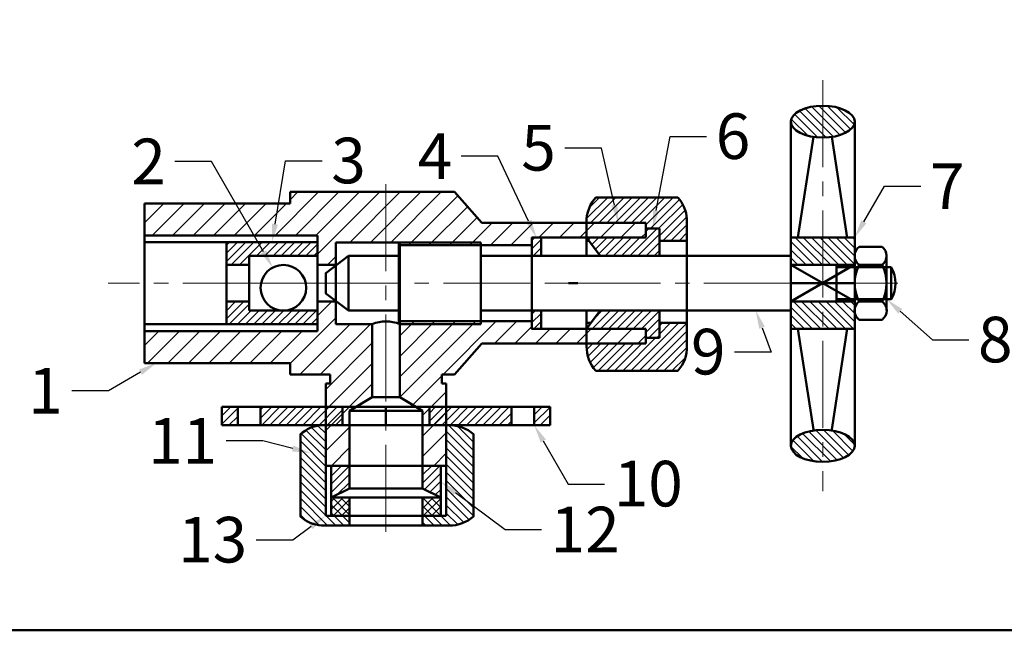
# Model space of a CAD drawing. Units: millimetres. Extents: x 123 to 731, y 468 to 864.
# Tile 2 of 5: x 328 to 544, y 468 to 602. Entities that reach past the tile are written whole.
import ezdxf
from ezdxf import colors
from ezdxf.entities.mleader import LeaderData, LeaderLine
from ezdxf.math import Vec2, Vec3

# ---------------------------------------------------------------- set-up
doc = ezdxf.new("R2010")
doc.units = ezdxf.units.MM
doc.linetypes.add('CENTER2', pattern=[28.575, 19.05, -3.175, 3.175, -3.175])
for name, color, linetype, lineweight in [('M-CNTR', 1, 'CENTER2', 18), ('M-HATC', 8, 'Continuous', 18), ('M-OUTL', 7, 'Continuous', 50), ('M-TEXT', 3, 'Continuous', 25)]:
    doc.layers.add(name, color=color, linetype=linetype, lineweight=lineweight)
doc.styles.get("Standard").update_dxf_attribs({"font": 'arial.ttf'})
pattern_1 = [(45, (-48.4416, -233.5905), (-0.8980256, 0.8980256), [])]
pattern_2 = [(135, (832.0712, 132.0536), (-0.8980256, -0.8980256), [])]
pattern_3 = [(45, (832.0712, 132.0536), (-0.8980256, 0.8980256), [])]

# ---------------------------------------------------------------- blocks, each defined once
blk = doc.blocks.new('*U26')
at = {"layer": 'M-CNTR', "color": 0, "transparency": 16777216}
blk.add_line((44.29, 0), (-105.45, 0), dxfattribs=at)
blk = doc.blocks.new('*U40')
at = {"layer": 'M-CNTR', "color": 0, "transparency": 16777216}
blk.add_line((6, 0), (-6, 0), dxfattribs=at)
blk = doc.blocks.new('*U42')
at = {"layer": 'M-CNTR', "color": 0, "transparency": 16777216}
blk.add_line((4.5, 0), (-4.5, 0), dxfattribs=at)
blk = doc.blocks.new('*U46')
at = {"layer": 'M-CNTR', "color": 0, "transparency": 16777216}
blk.add_line((0, -5.5), (0, 73.5), dxfattribs=at)
blk = doc.blocks.new('*U71')
at = {"layer": 'M-CNTR', "color": 0, "transparency": 16777216}
blk.add_line((13.5, 0), (-13.5, 0), dxfattribs=at)
blk = doc.blocks.new('*U83')
at = {"layer": 'M-CNTR', "color": 0, "transparency": 16777216}
blk.add_line((0, 53.48), (0, -36.6), dxfattribs=at)
blk = doc.blocks.new('HEX-NUT')
for p, q in [((6.02, 16), (1.02, 16)), ((1.02, 12), (6.02, 12)), ((1.02, 4), (6.02, 4)), ((1.02, 0), (6.02, 0))]:
    blk.add_line(p, q)
for centre, radius, start, end in [((2.47, 14), 2.47, 125.9888, 234.0112), ((4.57, 14), 2.47, 305.9888, 54.0112), ((8.52, 8), 8.5, 151.9275, 208.0725), ((-1.48, 8), 8.5, 331.9275, 28.0725), ((2.52, 2), 2.5, 126.8697, 233.1303), ((4.52, 2), 2.5, 306.8697, 53.1303)]:
    blk.add_arc(centre, radius, start, end)

msp = doc.modelspace()

# ---------------------------------------------------------------- hatches: boundary and pattern name
at = {"layer": 'M-HATC'}
h = msp.add_hatch(dxfattribs=at)
h.set_pattern_fill('ANSI31', color=256, scale=0.4, angle=-90)
h.set_pattern_definition([(315, (-204.5358, 1199.6268), (0.8980256, 0.8980256), [])])
edge = h.paths.add_edge_path()
edge.add_ellipse((504.0866, 579.9567), major_axis=(-7, 0), ratio=0.5, start_angle=90, end_angle=270)
edge.add_line((504.0866, 583.4567), (504.0866, 576.4567))
edge = h.paths.add_edge_path()
edge.add_ellipse((504.0866, 579.9567), major_axis=(-7, 0), ratio=0.5, start_angle=270, end_angle=450)
edge.add_line((504.0866, 576.4567), (504.0866, 583.4567))
h.paths.add_polyline_path([(511.0866, 548.5375), (511.0866, 554.5375), (504.0866, 554.5375), (504.0866, 548.5375)])
h.paths.add_polyline_path([(504.0866, 548.5375), (504.0866, 554.5375), (497.0866, 554.5375), (497.0866, 548.5375)])
h.paths.add_polyline_path([(511.0866, 534.5375), (511.0866, 540.5375), (504.0866, 540.5375), (504.0866, 534.5375)])
h.paths.add_polyline_path([(504.0866, 540.5375), (497.0866, 540.5375), (497.0866, 534.5375), (504.0866, 534.5375)])
edge = h.paths.add_edge_path()
edge.add_ellipse((504.0866, 508.902), major_axis=(-7, 0), ratio=0.5, start_angle=90, end_angle=270)
edge.add_line((504.0866, 512.402), (504.0866, 505.402))
edge = h.paths.add_edge_path()
edge.add_ellipse((504.0866, 508.902), major_axis=(-7, 0), ratio=0.5, start_angle=270, end_angle=450)
edge.add_line((504.0866, 505.402), (504.0866, 512.402))
h = msp.add_hatch(dxfattribs=at)
h.set_pattern_fill('ANSI31', color=256)
h.set_pattern_definition([(45, (832.0712, 132.0536), (-2.245064, 2.245064), [])])
h.paths.add_polyline_path([(411.2945, 519.5375), (416.2945, 516.5375), (416.2945, 504.5375), (421.5145, 504.5375), (421.5145, 522.5375), (420.5145, 522.5375), (420.5145, 524.5375), (423.2945, 524.5375), (429.2945, 531.3175), (440.2945, 531.3175), (465.2945, 531.3175), (465.2945, 534.5375), (440.2945, 534.5375), (440.2945, 536.2075), (411.2945, 536.2075), (411.2945, 535.5746)])
h.paths.add_polyline_path([(405.2945, 535.5746), (397.2945, 535.5746), (397.2945, 540.5375), (393.2945, 540.5375), (393.2945, 534.0575), (355.2945, 534.0575), (355.2945, 527.0375), (387.2945, 527.0375), (387.2945, 524.5375), (396.0745, 524.5375), (396.0745, 522.5375), (395.0745, 522.5375), (395.0745, 504.5375), (400.2945, 504.5375), (400.2945, 516.5375), (405.2945, 519.5375)])
h.paths.add_polyline_path([(387.2945, 564.5375), (387.2945, 562.0375), (355.2945, 562.0375), (355.2945, 555.0175), (393.2945, 555.0175), (393.2945, 548.5375), (397.2945, 548.5375), (397.2945, 553.5004), (411.2945, 553.5004), (411.2945, 552.8675), (440.2945, 552.8675), (440.2945, 554.5375), (465.2945, 554.5375), (465.2945, 557.7575), (440.2945, 557.7575), (429.2945, 557.7575), (423.2945, 564.5375)])
h = msp.add_hatch(dxfattribs=at)
h.set_pattern_fill('ANSI31', color=256, scale=0.4)
h.set_pattern_definition(pattern_3)
h.paths.add_polyline_path([(474.2945, 530.428), (474.2945, 535.8212), (468.2945, 535.8212), (468.2945, 532.5375), (465.2945, 532.5375), (465.2945, 531.3175), (452.2945, 531.3175), (452.2945, 530.428, 0.17944614), (454.2945, 525.3212), (472.2945, 525.3212, 0.17944614)])
h.paths.add_polyline_path([(472.2945, 563.3212), (454.2945, 563.3212, 0.16687276), (452.2945, 558.647), (452.2945, 557.7575), (465.2945, 557.7575), (465.2945, 556.5375), (468.2945, 556.5375), (468.2945, 553.8462), (474.2945, 553.8462), (474.2945, 558.647, 0.16687276)])
h = msp.add_hatch(dxfattribs=at)
h.set_pattern_fill('ANSI31', color=256, scale=0.4)
h.set_pattern_definition([(45, (-79.6213, -197.3759), (-0.8980256, 0.8980256), [])])
h.paths.add_polyline_path([(452.2945, 554.5375), (455.2945, 550.5375), (468.2945, 550.5375), (468.2945, 556.5375), (465.2945, 556.5375), (465.2945, 554.5375)])
h = msp.add_hatch(dxfattribs=at)
h.set_pattern_fill('ANSI31', color=256, scale=0.4)
h.set_pattern_definition([(45, (7.4622, -127.2527), (-0.8980256, 0.8980256), [])])
h.paths.add_polyline_path([(373.2945, 548.5375), (378.2945, 548.5375), (378.2945, 550.5375), (393.2945, 550.5375), (393.2945, 553.5375), (373.2945, 553.5375)])
h.paths.add_polyline_path([(393.2945, 535.5375), (393.2945, 538.5375), (378.2945, 538.5375), (378.2945, 540.5375), (373.2945, 540.5375), (373.2945, 535.5375)])
h = msp.add_hatch(dxfattribs=at)
h.set_pattern_fill('ANSI31', color=256, scale=0.4)
h.set_pattern_definition(pattern_3)
h.paths.add_polyline_path([(440.2945, 550.5375), (442.2945, 550.5375), (442.2945, 554.5375), (440.2945, 554.5375)])
h.paths.add_polyline_path([(442.2945, 538.5375), (440.2945, 538.5375), (440.2945, 534.5375), (442.2945, 534.5375)])
h = msp.add_hatch(dxfattribs=at)
h.set_pattern_fill('ANSI31', color=256, scale=0.4)
h.set_pattern_definition([(45, (-161.0183, -242.7467), (-0.8980256, 0.8980256), [])])
h.paths.add_polyline_path([(452.813, 553.8462), (452.2945, 554.5375), (452.2945, 553.8462)])
h = msp.add_hatch(dxfattribs=at)
h.set_pattern_fill('ANSI31', color=256, scale=0.4)
h.set_pattern_definition([(45, (835.1768, 97.1788), (-0.8980256, 0.8980256), [])])
h.paths.add_polyline_path([(455.2945, 538.5375), (452.2945, 534.5375), (465.2945, 534.5375), (465.2945, 532.5375), (468.2945, 532.5375), (468.2945, 538.5375)])
h = msp.add_hatch(dxfattribs=at)
h.set_pattern_fill('ANSI31', color=256, scale=0.4)
h.set_pattern_definition([(45, (834.237, 76.9075), (-0.8980256, 0.8980256), [])])
h.paths.add_polyline_path([(452.2945, 534.5375), (453.2574, 535.8212), (452.2945, 535.8212)])
h = msp.add_hatch(dxfattribs=at)
h.set_pattern_fill('ANSI31', color=256, scale=0.4)
h.set_pattern_definition([(45, (-72.056, -58.2177), (-0.8980256, 0.8980256), [])])
h.paths.add_polyline_path([(375.7945, 517.4172), (372.2945, 517.4172), (372.2945, 513.4172), (375.7945, 513.4172)])
h.paths.add_polyline_path([(398.7695, 513.4172), (398.7695, 517.4172), (380.7945, 517.4172), (380.7945, 513.4172)])
h.paths.add_polyline_path([(435.7945, 513.4172), (435.7945, 517.4172), (417.8195, 517.4172), (417.8195, 513.4172)])
h.paths.add_polyline_path([(440.7945, 513.4172), (444.2945, 513.4172), (444.2945, 517.4172), (440.7945, 517.4172)])
h = msp.add_hatch(dxfattribs=at)
h.set_pattern_fill('ANSI31', color=256, scale=0.4, angle=90)
h.set_pattern_definition(pattern_2)
h.paths.add_polyline_path([(395.0745, 504.5375), (395.0745, 513.4172), (394.1851, 513.4172, 0.16687276), (389.5108, 511.4172), (389.5108, 493.4172, 0.16687276), (394.1851, 491.4172), (400.2945, 491.4172), (400.2945, 493.5375), (396.2945, 493.5375), (395.0745, 493.5375)])
h.paths.add_polyline_path([(421.5145, 493.5375), (420.2945, 493.5375), (416.2945, 493.5375), (416.2945, 491.4172), (422.404, 491.4172, 0.17944614), (427.5108, 493.4172), (427.5108, 511.4172, 0.20874254), (421.5145, 513.3831), (421.5145, 504.5375)])
h = msp.add_hatch(dxfattribs=at)
h.set_pattern_fill('ANSI31', color=256, scale=0.4)
h.set_pattern_definition([(45, (926.4336, -118.8602), (-0.8980256, 0.8980256), [])])
h.paths.add_polyline_path([(400.2945, 504.5375), (396.2945, 504.5375), (396.2945, 497.5375), (400.2945, 499.5375)])
h.paths.add_polyline_path([(420.2945, 504.5375), (416.2945, 504.5375), (416.2945, 499.5375), (420.2945, 497.5375)])
h = msp.add_hatch(dxfattribs=at)
h.set_pattern_fill('ANSI31', color=256, scale=0.4)
h.set_pattern_definition(pattern_1)
h.paths.add_polyline_path([(396.2945, 497.5375), (400.2945, 497.5375), (400.2945, 493.5375), (396.2945, 493.5375)])
h = msp.add_hatch(dxfattribs=at)
h.set_pattern_fill('ANSI31', color=256, scale=0.4, angle=90)
h.set_pattern_definition(pattern_2)
h.paths.add_polyline_path([(400.2945, 497.5375), (396.2945, 497.5375), (396.2945, 493.5375), (400.2945, 493.5375)])
h.paths.add_polyline_path([(420.2945, 497.5375), (416.2945, 497.5375), (416.2945, 493.5375), (420.2945, 493.5375)])
h = msp.add_hatch(dxfattribs=at)
h.set_pattern_fill('ANSI31', color=256, scale=0.4)
h.set_pattern_definition(pattern_1)
h.paths.add_polyline_path([(416.2945, 493.5375), (420.2945, 493.5375), (420.2945, 497.5375), (416.2945, 497.5375)])

# ---------------------------------------------------------------- linework, layer by layer
at = {"layer": 'M-OUTL'}
for p, q in [((497.0866, 544.5375), (497.0866, 579.9567)), ((511.0866, 579.9567), (511.0866, 508.902)), ((502.0866, 576.6026), (498.615, 554.5375)), ((506.0873, 576.5936), (509.4596, 554.5131)), ((387.2945, 562.0375), (387.2945, 564.5375)), ((387.2945, 564.5375), (423.2945, 564.5375)), ((429.2945, 557.7575), (423.2945, 564.5375)), ((355.2945, 562.0375), (355.2945, 555.0175)), ((355.2945, 562.0375), (387.2945, 562.0375)), ((472.2945, 563.3212), (454.2945, 563.3212)), ((440.2945, 557.7575), (429.2945, 557.7575)), ((465.2945, 557.7575), (440.2945, 557.7575)), ((452.2945, 558.647), (452.2945, 550.5375)), ((465.2945, 556.5375), (465.2945, 557.7575)), ((474.2945, 530.428), (474.2945, 558.647)), ((393.2945, 555.0175), (355.2945, 555.0175)), ((355.2945, 555.0175), (355.2945, 534.0575)), ((393.2945, 555.0175), (393.2945, 548.5375)), ((468.2945, 556.5375), (465.2945, 556.5375)), ((465.2945, 556.5375), (465.2945, 554.5375)), ((468.2945, 550.5375), (468.2945, 556.5375)), ((373.2945, 553.5375), (355.2945, 553.5375)), ((373.2945, 553.5375), (373.2945, 535.5375)), ((393.2945, 553.5375), (373.2945, 553.5375)), ((393.2945, 535.5375), (393.2945, 553.5375)), ((397.2945, 553.5004), (397.2945, 535.5746)), ((411.2945, 553.5004), (397.2945, 553.5004)), ((411.0866, 553.5004), (411.0866, 535.5746)), ((429.0866, 553.5004), (411.0866, 553.5004)), ((411.2945, 553.5004), (411.2945, 544.5375)), ((440.2945, 552.8675), (411.2945, 552.8675)), ((411.2945, 544.5375), (411.2945, 552.8675)), ((440.2945, 554.5375), (440.2945, 534.5375)), ((465.2945, 554.5375), (440.2945, 554.5375)), ((452.2945, 554.5375), (452.2945, 550.5375)), ((465.2945, 554.5375), (452.2945, 554.5375)), ((455.2945, 550.5375), (452.2945, 554.5375)), ((452.2945, 553.8462), (452.813, 553.8462)), ((452.2945, 550.5375), (452.2945, 553.8462)), ((468.2945, 553.8462), (474.2945, 553.8462)), ((497.0866, 554.5375), (511.0866, 554.5375)), ((511.0866, 550.8457), (511.0866, 538.5333)), ((518.0866, 538.5333), (518.0866, 550.8457)), ((373.2945, 548.5375), (378.2945, 548.5375)), ((393.2945, 550.5375), (378.2945, 550.5375)), ((378.2945, 550.5375), (378.2945, 538.5375)), ((397.2945, 548.5375), (393.2945, 548.5375)), ((393.2945, 548.5375), (393.2945, 540.5375)), ((397.2945, 548.5375), (397.2945, 540.5375)), ((411.0866, 550.5375), (400.0866, 550.5375)), ((448.3346, 550.5375), (450.3346, 550.5375)), ((452.2945, 550.5375), (468.2945, 550.5375)), ((497.0866, 548.5375), (511.0866, 548.5375)), ((497.0866, 540.5375), (510.943, 548.5375)), ((497.0866, 548.5375), (511.0866, 540.5375)), ((411.2945, 544.5375), (411.2945, 536.2075)), ((411.2945, 535.5746), (411.2945, 544.5375)), ((448.3346, 544.5375), (450.3346, 544.5375)), ((497.0866, 508.902), (497.0866, 544.5375)), ((497.0866, 544.5375), (511.0866, 544.5375)), ((373.2945, 540.5375), (378.2945, 540.5375)), ((393.2945, 540.5375), (397.2945, 540.5375)), ((393.2945, 534.0575), (393.2945, 540.5375)), ((497.0866, 540.5375), (511.0866, 540.5375)), ((378.2945, 538.5375), (393.2945, 538.5375)), ((448.3346, 538.5375), (450.3346, 538.5375)), ((452.2945, 538.5375), (468.2945, 538.5375)), ((452.2945, 534.5375), (455.2945, 538.5375)), ((452.2945, 538.5375), (452.2945, 530.428)), ((452.2945, 538.5375), (452.2945, 534.5375)), ((468.2945, 532.5375), (468.2945, 538.5375)), ((405.2945, 535.5746), (397.2945, 535.5746)), ((405.2945, 535.5746), (405.2945, 519.5375)), ((440.2945, 536.2075), (411.2945, 536.2075)), ((411.2945, 535.5746), (411.2945, 519.5375)), ((429.0866, 535.5746), (411.2945, 535.5746)), ((452.2945, 535.8212), (453.2574, 535.8212)), ((468.2945, 535.8212), (474.2945, 535.8212)), ((373.2945, 535.5375), (355.2945, 535.5375)), ((355.2945, 534.0575), (393.2945, 534.0575)), ((355.2945, 527.0375), (355.2945, 534.0575)), ((373.2945, 535.5375), (393.2945, 535.5375)), ((465.2945, 534.5375), (440.2945, 534.5375)), ((452.2945, 534.5375), (465.2945, 534.5375)), ((465.2945, 534.5375), (465.2945, 532.5375)), ((497.0866, 534.5375), (511.0866, 534.5375)), ((502.0866, 512.4723), (498.615, 534.5375)), ((506.0873, 512.4813), (509.4596, 534.5619)), ((429.2945, 531.3175), (423.2945, 524.5375)), ((440.2945, 531.3175), (429.2945, 531.3175)), ((465.2945, 531.3175), (440.2945, 531.3175)), ((465.2945, 531.3175), (440.2945, 531.3175)), ((465.2945, 532.5375), (468.2945, 532.5375)), ((465.2945, 531.3175), (465.2945, 532.5375)), ((355.2945, 527.0375), (387.2945, 527.0375)), ((387.2945, 527.0375), (387.2945, 524.5375)), ((454.2945, 525.3212), (472.2945, 525.3212)), ((387.2945, 524.5375), (396.0745, 524.5375)), ((395.0745, 524.5375), (396.0745, 524.5375)), ((396.0745, 524.5375), (396.0745, 522.5375)), ((420.5145, 524.5375), (420.5145, 522.5375)), ((420.5145, 524.5375), (423.2945, 524.5375)), ((395.0745, 504.5375), (395.0745, 522.5375)), ((396.0745, 522.5375), (395.0745, 522.5375)), ((420.5145, 522.5375), (421.5145, 522.5375)), ((421.5145, 504.5375), (421.5145, 522.5375)), ((405.2945, 519.5375), (400.2945, 516.5375)), ((405.2945, 519.5375), (411.2945, 519.5375)), ((411.2945, 519.5375), (416.2945, 516.5375)), ((444.2945, 517.4172), (372.2945, 517.4172)), ((372.2945, 517.4172), (372.2945, 513.4172)), ((375.7945, 513.4172), (375.7945, 517.4172)), ((380.7945, 513.4172), (380.7945, 517.4172)), ((398.7695, 517.4172), (398.7695, 513.4172)), ((416.2945, 516.5375), (400.2945, 516.5375)), ((400.2945, 516.5375), (400.2945, 504.5375)), ((408.2945, 517.4172), (408.2945, 513.4172)), ((416.2945, 504.5375), (416.2945, 516.5375)), ((417.8195, 517.4172), (417.8195, 513.4172)), ((435.7945, 513.4172), (435.7945, 517.4172)), ((440.7945, 513.4172), (440.7945, 517.4172)), ((444.2945, 513.4172), (444.2945, 517.4172)), ((372.2945, 513.4172), (444.2945, 513.4172)), ((408.2945, 504.5375), (395.0745, 504.5375)), ((395.0745, 504.5375), (395.0745, 493.5375)), ((420.2945, 504.5375), (396.2945, 504.5375)), ((396.2945, 504.5375), (396.2945, 497.5375)), ((400.2945, 504.5375), (416.2945, 504.5375)), ((400.2945, 504.5375), (400.2945, 499.5375)), ((408.2945, 504.5375), (421.5145, 504.5375)), ((416.2945, 504.5375), (416.2945, 499.5375)), ((420.2945, 497.5375), (420.2945, 504.5375)), ((421.5145, 504.5375), (421.5145, 493.5375)), ((400.2945, 499.5375), (396.2945, 497.5375)), ((400.2945, 499.5375), (408.2945, 499.5375)), ((416.2945, 499.5375), (408.2945, 499.5375)), ((416.2945, 499.5375), (420.2945, 497.5375)), ((420.2945, 497.5375), (396.2945, 497.5375)), ((396.2945, 497.5375), (396.2945, 493.5375)), ((396.2945, 497.5375), (420.2945, 497.5375)), ((400.2945, 497.5375), (400.2945, 493.5375)), ((416.2945, 497.5375), (416.2945, 493.5375)), ((420.2945, 493.5375), (420.2945, 497.5375)), ((396.2945, 493.5375), (395.0745, 493.5375)), ((396.2945, 493.5375), (420.2945, 493.5375)), ((400.2945, 493.5375), (400.2945, 491.4172)), ((416.2945, 493.5375), (416.2945, 491.4172)), ((420.2945, 493.5375), (421.5145, 493.5375))]:
    msp.add_line(p, q, dxfattribs=at)
msp.add_lwpolyline([(123.3719, 863.9604), (731.4761, 863.9604), (731.4761, 468.4518), (123.3719, 468.4518)], close=True, dxfattribs=at)
for points in [[(411.0866, 553.5004), (411.0866, 535.5746)], [(429.0866, 535.5746), (429.0866, 553.5004)], [(442.2945, 550.5375), (442.2945, 554.5375), (440.2945, 554.5375), (440.2945, 550.5375)], [(400.0866, 538.5375), (400.0866, 550.5375), (395.0866, 546.7697), (395.0866, 542.3052), (400.0866, 538.5375), (411.0866, 538.5375)], [(429.0866, 550.5375), (497.0866, 550.5375), (497.0866, 538.5375), (429.0866, 538.5375)], [(497.0866, 548.5375), (507.0866, 548.5375), (507.0866, 540.5375), (497.0866, 540.5375)], [(507.0866, 548.0375), (519.0866, 548.0375), (519.0866, 541.0375), (507.0866, 541.0375)], [(440.2945, 538.5375), (440.2945, 534.5375), (442.2945, 534.5375), (442.2945, 538.5375)]]:
    msp.add_lwpolyline(points, dxfattribs=at)
for points in [[(422.404, 513.4172), (394.1851, 513.4172, 0.16687276), (389.5108, 511.4172), (389.5108, 493.4172, 0.16687276), (394.1851, 491.4172), (422.404, 491.4172)], [(422.1175, 491.4172, 0.18883672), (427.5108, 493.4172), (427.5108, 511.4172, 0.18883672), (422.1175, 513.4172)]]:
    msp.add_lwpolyline(points, format="xyb", dxfattribs=at)
msp.add_circle((385.7945, 543.5375), 5, dxfattribs=at)
for centre, radius, start, end in [((460.1023, 558.0712), 7.829, 137.887598, 175.782841), ((466.4868, 558.0712), 7.829, 4.217159, 42.112402), ((513.0244, 544.5375), 7, 330, 30), ((408.2945, 528.0295), 8.1196, 68.316751, 111.683249), ((460.18, 530.5712), 7.8868, 178.959216, 221.733715), ((466.409, 530.5712), 7.8868, 318.266285, 1.040784)]:
    msp.add_arc(centre, radius, start, end, dxfattribs=at)
for centre in [(504.0866, 579.9567), (504.0866, 508.902)]:
    msp.add_ellipse(centre, major_axis=(-7, 0), ratio=0.5, dxfattribs=at)

# ---------------------------------------------------------------- block references
at = {"layer": 'M-CNTR'}
for name, p in [('*U83', (504.0866, 535.5745)), ('*U46', (408.2945, 495.5375)), ('*U26', (452.7945, 544.5375)), ('*U71', (383.2945, 544.5375)), ('*U42', (449.3346, 544.5375)), ('*U40', (514.5866, 544.5375))]:
    msp.add_blockref(name, p, dxfattribs=at)
at = {"layer": 'M-OUTL', "rotation": 180}
msp.add_blockref('HEX-NUT', (518.1055, 552.5371), dxfattribs=at)

# ---------------------------------------------------------------- leaders
at = {"layer": 'M-TEXT'}
ml = msp.add_multileader_mtext('Standard', dxfattribs=at)
ml.set_content('6', color=256)
ml.set_leader_properties()
ml.build(insert=Vec2(0, 0))
ctx = ml.context
ctx.base_point, ctx.char_height, ctx.plane_origin = Vec3(478.617, 576.688), 10, Vec3(466.7945, 556.5375)
notes = []
notes.append((ctx, [(0, (1, 1, 0), (470.617, 576.688), (1, 0), 8, [(0, [(466.7945, 556.5375)], 0, [])])]))
ctx.mtext.insert, ctx.mtext.flow_direction = Vec3(480.617, 581.7732), 5
ml = msp.add_multileader_mtext('Standard', dxfattribs=at)
ml.set_content('5', color=256)
ml.set_leader_properties()
ml.build(insert=Vec2(0, 0))
ctx = ml.context
ctx.base_point, ctx.char_height, ctx.plane_origin = Vec3(436.9076, 574.1439), 10, Vec3(459.2795, 557.7575)
ctx.text_align_type = 2
notes.append((ctx, [(0, (1, 1, 0), (455.5379, 574.1439), (-1, 0), 8, [(0, [(459.2795, 557.7575)], 0, [])])]))
ctx.mtext.insert, ctx.mtext.alignment, ctx.mtext.flow_direction = Vec3(445.5379, 579.2292), 3, 5
ml = msp.add_multileader_mtext('Standard', dxfattribs=at)
ml.set_content('3', color=256)
ml.set_leader_properties()
ml.build(insert=Vec2(0, 0))
ctx = ml.context
ctx.base_point, ctx.char_height, ctx.plane_origin = Vec3(394.2877, 571.3496), 10, Vec3(383.2945, 553.5375)
notes.append((ctx, [(0, (1, 1, 0), (386.2877, 571.3496), (1, 0), 8, [(0, [(383.2945, 553.5375)], 0, [])])]))
ctx.mtext.insert, ctx.mtext.flow_direction = Vec3(396.2877, 576.4383), 5
ml = msp.add_multileader_mtext('Standard', dxfattribs=at)
ml.set_content('4', color=256)
ml.set_leader_properties()
ml.build(insert=Vec2(0, 0))
ctx = ml.context
ctx.base_point, ctx.char_height, ctx.plane_origin = Vec3(413.8827, 572.4011), 10, Vec3(441.2945, 554.5375)
ctx.text_align_type = 2
notes.append((ctx, [(0, (1, 1, 0), (432.7995, 572.4011), (-1, 0), 8, [(0, [(441.2945, 554.5375)], 0, [])])]))
ctx.mtext.insert, ctx.mtext.alignment, ctx.mtext.flow_direction = Vec3(422.7995, 577.4011), 3, 5
ml = msp.add_multileader_mtext('Standard', dxfattribs=at)
ml.set_content('2', color=256)
ml.set_leader_properties()
ml.build(insert=Vec2(0, 0))
ctx = ml.context
ctx.base_point, ctx.char_height, ctx.plane_origin = Vec3(351.3878, 571.2418), 10, Vec3(383.4551, 547.9564)
ctx.text_align_type = 2
notes.append((ctx, [(0, (1, 1, 0), (370.0113, 571.2418), (-1, 0), 8, [(0, [(383.4551, 547.9564)], 0, [])])]))
ctx.mtext.insert, ctx.mtext.alignment, ctx.mtext.flow_direction = Vec3(360.0113, 576.2418), 3, 5
ml = msp.add_multileader_mtext('Standard', dxfattribs=at)
ml.set_content('7', color=256)
ml.set_leader_properties()
ml.build(insert=Vec2(0, 0))
ctx = ml.context
ctx.base_point, ctx.char_height, ctx.plane_origin = Vec3(525.5978, 565.8151), 10, Vec3(511.0866, 554.5375)
notes.append((ctx, [(0, (1, 1, 0), (517.5978, 565.8151), (1, 0), 8, [(0, [(511.0866, 554.5375)], 0, [])])]))
ctx.mtext.insert, ctx.mtext.flow_direction = Vec3(527.5978, 570.8151), 5
ml = msp.add_multileader_mtext('Standard', dxfattribs=at)
ml.set_content('8', color=256)
ml.set_leader_properties()
ml.build(insert=Vec2(0, 0))
ctx = ml.context
ctx.base_point, ctx.char_height, ctx.plane_origin = Vec3(536.1336, 532.1043), 10, Vec3(518.0866, 541.0375)
notes.append((ctx, [(0, (1, 1, 0), (528.1336, 532.1043), (1, 0), 8, [(0, [(518.0866, 541.0375)], 0, [])])]))
ctx.mtext.insert, ctx.mtext.flow_direction = Vec3(538.1336, 537.1896), 5
ml = msp.add_multileader_mtext('Standard', dxfattribs=at)
ml.set_content('9', color=256)
ml.set_leader_properties()
ml.build(insert=Vec2(0, 0))
ctx = ml.context
ctx.base_point, ctx.char_height, ctx.plane_origin = Vec3(474.1772, 529.4592), 10, Vec3(489.3806, 538.5375)
ctx.text_align_type = 2
notes.append((ctx, [(0, (1, 1, 0), (492.7529, 529.4592), (-1, 0), 8, [(0, [(489.3806, 538.5375)], 0, [])])]))
ctx.mtext.insert, ctx.mtext.alignment, ctx.mtext.flow_direction = Vec3(482.7529, 534.5445), 3, 5
ml = msp.add_multileader_mtext('Standard', dxfattribs=at)
ml.set_content('1', color=256)
ml.set_leader_properties()
ml.build(insert=Vec2(0, 0))
ctx = ml.context
ctx.base_point, ctx.char_height, ctx.plane_origin = Vec3(331.7242, 520.9738), 10, Vec3(357.9103, 527.0375)
ctx.text_align_type = 2
notes.append((ctx, [(0, (1, 1, 0), (347.4077, 520.9738), (-1, 0), 8, [(0, [(357.9103, 527.0375)], 0, [])])]))
ctx.mtext.insert, ctx.mtext.alignment, ctx.mtext.flow_direction = Vec3(337.4077, 525.9738), 3, 5
ml = msp.add_multileader_mtext('Standard', dxfattribs=at)
ml.set_content('11', color=256)
ml.set_leader_properties()
ml.build(insert=Vec2(0, 0))
ctx = ml.context
ctx.base_point, ctx.char_height, ctx.plane_origin = Vec3(357.8133, 509.969), 10, Vec3(391.7067, 507.3337)
ctx.text_align_type = 2
notes.append((ctx, [(0, (1, 1, 0), (381.2663, 509.969), (-1, 0), 8, [(0, [(391.7067, 507.3337)], 0, [])])]))
ctx.mtext.insert, ctx.mtext.alignment, ctx.mtext.flow_direction = Vec3(371.2663, 514.969), 3, 5
ml = msp.add_multileader_mtext('Standard', dxfattribs=at)
ml.set_content('10', color=256)
ml.set_leader_properties()
ml.build(insert=Vec2(0, 0))
ctx = ml.context
ctx.base_point, ctx.char_height, ctx.plane_origin = Vec3(456.2402, 500.5209), 10, Vec3(440.7945, 513.4172)
notes.append((ctx, [(0, (1, 1, 0), (448.2402, 500.5209), (1, 0), 8, [(0, [(440.7945, 513.4172)], 0, [])])]))
ctx.mtext.insert, ctx.mtext.flow_direction = Vec3(458.2402, 505.6062), 5
ml = msp.add_multileader_mtext('Standard', dxfattribs=at)
ml.set_content('12', color=256)
ml.set_leader_properties()
ml.build(insert=Vec2(0, 0))
ctx = ml.context
ctx.base_point, ctx.char_height, ctx.plane_origin = Vec3(442.404, 490.5344), 10, Vec3(420.2945, 501.0375)
notes.append((ctx, [(0, (1, 1, 0), (434.404, 490.5344), (1, 0), 8, [(0, [(420.2945, 501.0375)], 0, [])])]))
ctx.mtext.insert, ctx.mtext.flow_direction = Vec3(444.404, 495.5344), 5
ml = msp.add_multileader_mtext('Standard', dxfattribs=at)
ml.set_content('13', color=256)
ml.set_leader_properties()
ml.build(insert=Vec2(0, 0))
ctx = ml.context
ctx.base_point, ctx.char_height, ctx.plane_origin = Vec3(362.457, 488.2273), 10, Vec3(395.0745, 493.5375)
ctx.text_align_type = 2
notes.append((ctx, [(0, (1, 1, 0), (387.8403, 488.2273), (-1, 0), 8, [(0, [(395.0745, 493.5375)], 0, [])])]))
ctx.mtext.insert, ctx.mtext.alignment, ctx.mtext.flow_direction = Vec3(377.8403, 493.316), 3, 5
for ctx, leaders in notes:
    for number, flags, end, landing, length, lines in leaders:
        leader = LeaderData()
        leader.index, (leader.has_last_leader_line, leader.has_dogleg_vector, leader.attachment_direction) = number, flags
        leader.last_leader_point, leader.dogleg_vector, leader.dogleg_length = Vec3(end), Vec3(landing), length
        for number, points, colour, breaks in lines:
            line = LeaderLine()
            line.index, line.vertices, line.color, line.breaks = number, Vec3.list(points), colors.encode_raw_color(colour), breaks
            leader.lines.append(line)
        ctx.leaders.append(leader)

doc.saveas('drawing.dxf')
